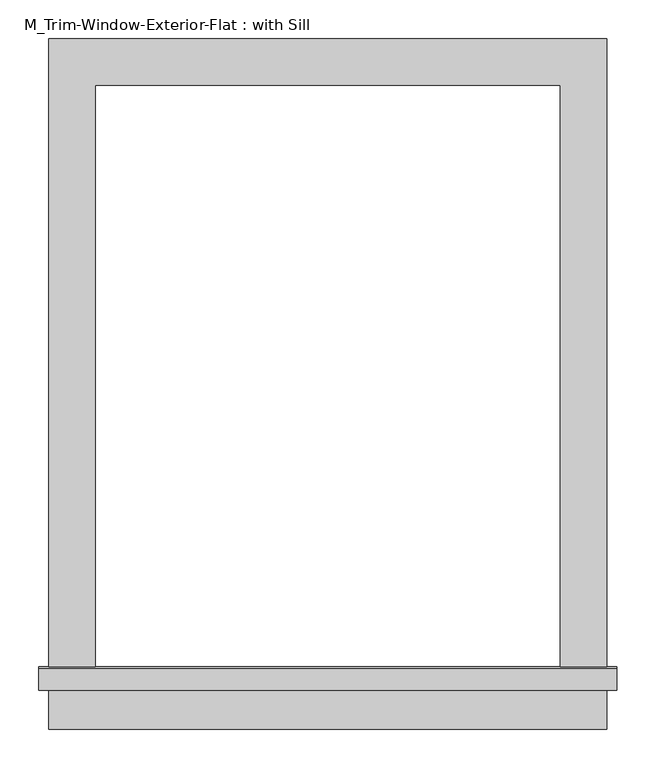
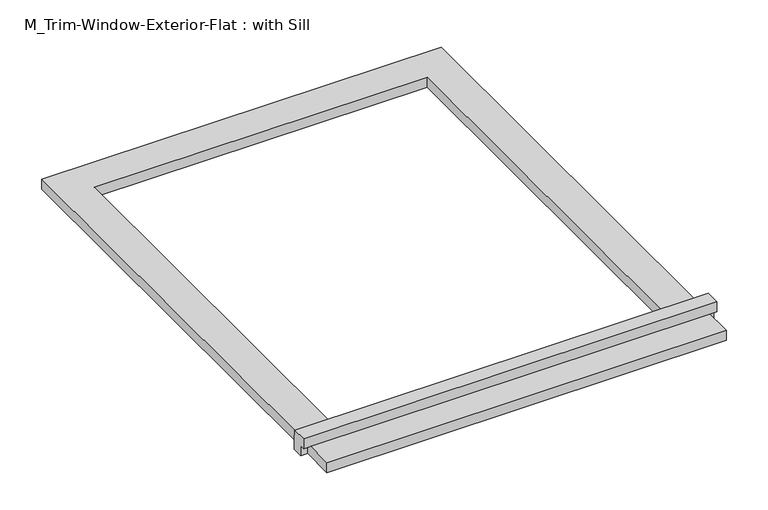
"""IFC4 building model written with IfcOpenShell, lengths in millimetres: proxy geometry, M_Trim-Window-Exterior-Flat : with Sill."""

from ifc_helpers import new_model, si_unit, frame, origin, origin_with_axes, place, context, project, spatial, polyline, outline, extrude, source, transform, mapped, element, save


def m_trim_window_exterior_flat_with_sill_a736bdd3(model_context):
    return source(origin(), model_context, "Body", "SweptSolid", [
        extrude(outline(polyline([(360.0, -770.4323709), (360.0, -830.4323709), (-360.0, -830.4323709), (-360.0, -770.4323709), (360.0, -770.4323709)])), origin_with_axes(), (0.0, 0.0, 1.0), 19.05),
        extrude(outline(polyline([(-780.0, 38.1), (-752.4580645, 38.1), (-750.0, 19.05), (-750.0, 0.0), (-770.4323709, 0.0), (-770.4323709, 19.05), (-780.0, 19.05), (-780.0, 38.1)])), frame((-372.7, 0.0, 0.0), z_axis=(1.0, 0.0, 0.0), x_axis=(0.0, 1.0, 0.0)), (0.0, 0.0, 1.0), 745.4),
        extrude(outline(polyline([(-360.0, 60.0), (360.0, 60.0), (360.0, -750.0), (300.0, -750.0), (300.0, 0.0), (-300.0, 0.0), (-300.0, -750.0), (-360.0, -750.0), (-360.0, 60.0)])), origin_with_axes(), (0.0, 0.0, 1.0), 19.05),
    ])


if __name__ == "__main__":
    model = new_model("IFC4")
    model_context = context("Model", 3, world=origin())
    ifc_project = project(units=[si_unit("LENGTHUNIT", "METRE", prefix="MILLI")], contexts=[model_context])
    site = spatial("IfcSite", under=ifc_project)
    building = spatial("IfcBuilding", under=site)
    placement = place(None, origin())
    m_trim_window_exterior_flat_with_sill_shape = m_trim_window_exterior_flat_with_sill_a736bdd3(model_context)
    element("IfcBuildingElementProxy", 1, Name="M_Trim-Window-Exterior-Flat : with Sill", ObjectType="M_Trim-Window-Exterior-Flat : with Sill", at=placement, inside=building, context=model_context, shape_type="MappedRepresentation", body=[
        mapped(m_trim_window_exterior_flat_with_sill_shape, transform((0.0, 0.0, 0.0), x_axis=(1.0, 0.0, 0.0), y_axis=(0.0, 1.0, 0.0), z_axis=(0.0, 0.0, 1.0))),
    ])
    save(model, "model.ifc")

# Revit data of these elements
# Type "M_Trim-Window-Exterior-Flat : with Sill"
#   Trim Width = 0.06 m
#   Trim Thickness_Picture Frame = 0.03 m
#   Trim Thickness_with Sill = 0.01905 m
#   Sill Thickness = 0.03 m
#   Opening Width [instance default] = 0.6 m
#   Opening Height [instance default] = 0.9 m
#   Default Elevation = 1.2 m
#   Sill = yes
#   Picture Frame = no
#   Trim Material [instance default] = none
# Element 1 (IfcBuildingElementProxy, "M_Trim-Window-Exterior-Flat : with Sill")
#   Opening Height = 0.75 m
#   Trim Material = Clad - White
#   Materials on its faces: "Clad - White"
# Materials
#   "Clad - White": class "Wood", colour RGB 242 242 238, transparency 0, Cost = 0
